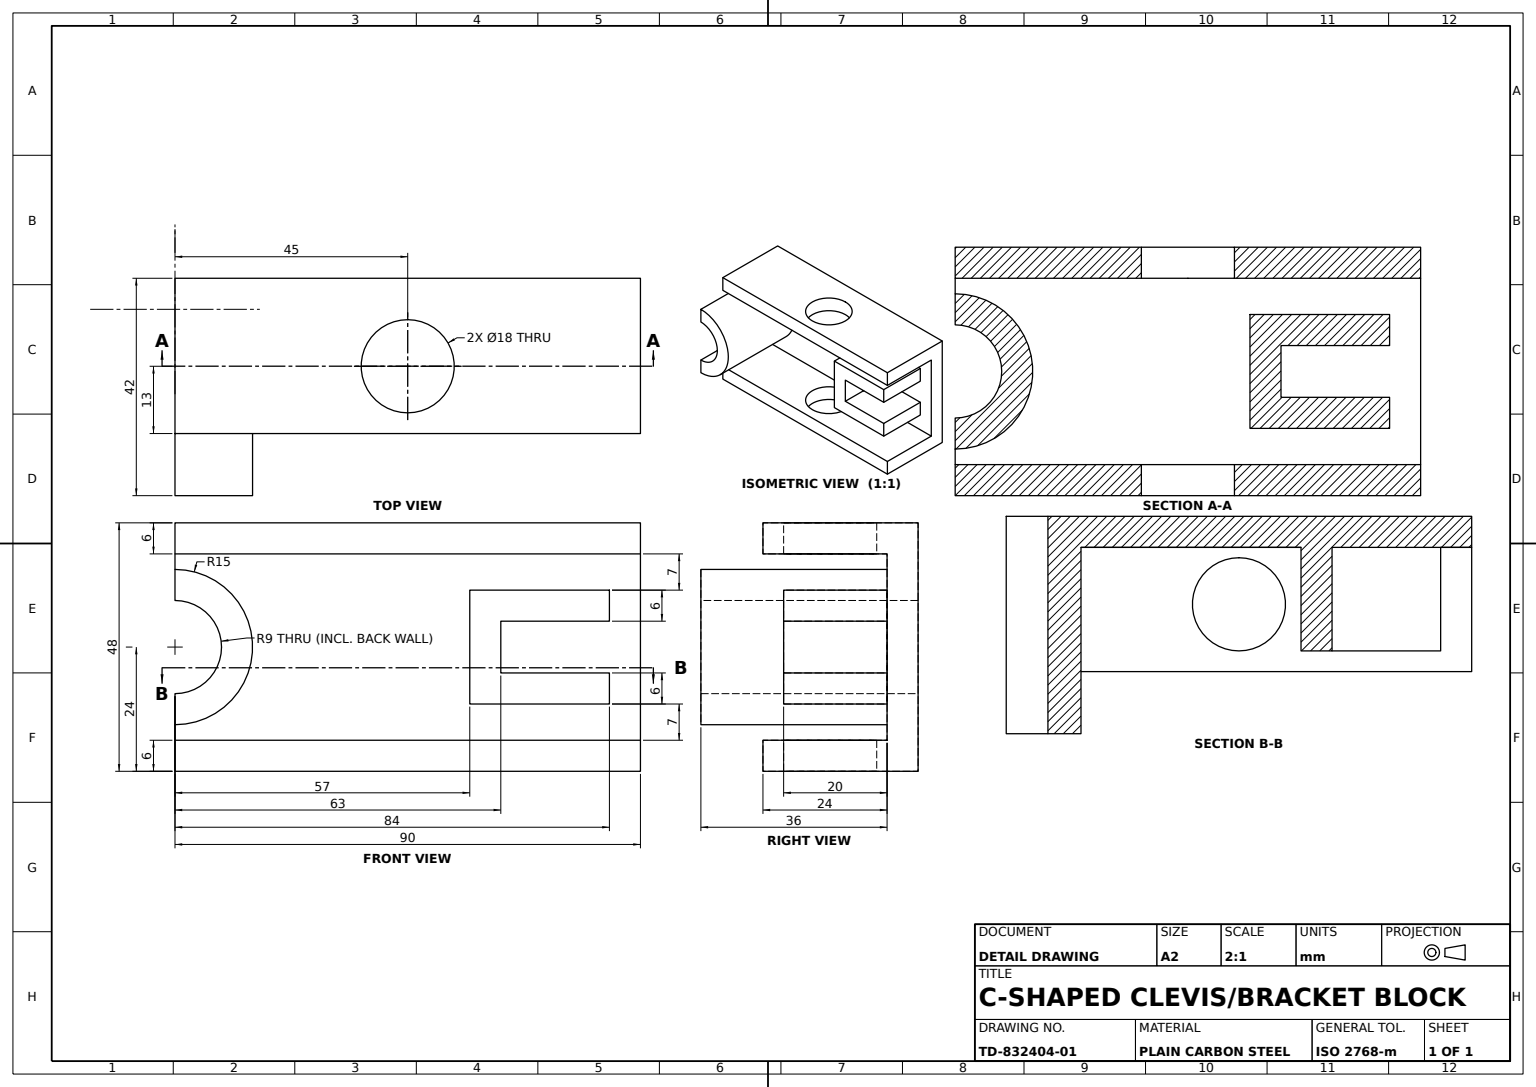
SolidWorks part; units mm, degrees
material "Plain Carbon Steel"
ref_plane "Front Plane" through (0, 0, 0) normal (0, 0, 1) x (1, 0, 0)
ref_plane "Top Plane" through (0, 0, 0) normal (0, 1, 0) x (1, 0, 0)
ref_plane "Right Plane" through (0, 0, 0) normal (1, 0, 0) x (0, 0, -1)
sketch "Base Block Sketch" plane through (0, 0, 0) normal (0, 0, 1) x (1, 0, 0)
  line L0 (0, 0) -> (90, 0)
  line L1 (90, 0) -> (90, 48)
  line L2 (90, 48) -> (0, 48)
  line L3 (0, 48) -> (0, 0)
  dimension "D1" = 90
  dimension "D2" = 48
extrude "Base Block" add sketch "Base Block Sketch" along normal blind 30
sketch "Channel Slot Sketch" plane through (0, 0, 30) normal (0, 0, 1) x (1, 0, 0)
  line L0 (6, 42) -> (6, 6)
  line L1 (0, 48) -> (0, 0) construction
  line L2 (0, 0) -> (90, 0) construction
  line L8 (84, 42) -> (6, 42)
  line L10 (6, 6) -> (84, 6)
  line L11 (84, 6) -> (84, 42)
  dimension "D1" = 6
  dimension "D2" = 84
  dimension "D3" = 6
  dimension "D4" = 42
extrude "Channel Slot" cut sketch "Channel Slot Sketch" against normal blind 24
sketch "Channel Relief Cut 1 Sketch" plane through (0, 0, 30) normal (0, 0, 1) x (1, 0, 0)
  line L0 (6, 42) -> (0, 42)
  line L1 (0, 48) -> (0, 0) construction
  line L2 (0, 42) -> (0, 6)
  line L3 (0, 6) -> (6, 6)
  line L4 (6, 6) -> (6, 42)
extrude "Channel Relief Cut 1" cut sketch "Channel Relief Cut 1 Sketch" against normal blind 24
sketch "Channel Relief Cut 2 Sketch" plane through (0, 0, 30) normal (0, 0, 1) x (1, 0, 0)
  line L0 (84, 42) -> (84, 6)
  line L1 (84, 6) -> (90, 6)
  line L2 (90, 0) -> (90, 48) construction
  line L3 (90, 6) -> (90, 42)
  line L4 (90, 42) -> (84, 42)
extrude "Channel Relief Cut 2" cut sketch "Channel Relief Cut 2 Sketch" against normal blind 24
sketch "Half Cylinder Boss Sketch" plane through (0, 0, 6) normal (0, 0, 1) x (1, 0, 0)
  line L0 (0, 42) -> (0, 6) construction
  line L1 (0, 39) -> (0, 9)
  arc A0 (0, 9) -> (0, 39) centre (0, 24) ccw
  dimension "D1" = 30
  dimension "D2" = 15
extrude "Half Cylinder Boss" add sketch "Half Cylinder Boss Sketch" along normal blind 36
sketch "Boss Bore Sketch" plane through (0, 0, 42) normal (0, 0, 1) x (1, 0, 0)
  line L0 (0, 39) -> (0, 9) construction
  line L1 (0, 33) -> (0, 15)
  arc A0 (0, 15) -> (0, 33) centre (0, 24) ccw
  dimension "D1" = 18
  dimension "D2" = 9
extrude "Boss Bore Ø18" cut sketch "Boss Bore Sketch" against normal blind 42
sketch "Upper Plate Hole Sketch" plane through (0, 0, 0) normal (0, -1, 0) x (1, 0, 0)
  line L0 (0, 30) -> (90, 30) construction
  line L1 (90, 30) -> (90, 0) construction
  circle A0 centre (45, 17) radius 9
  dimension "D1" = 18
  dimension "D4" = 18
  dimension "D2" = 13
  dimension "D3" = 45
extrude "Upper Plate Hole Ø18" cut sketch "Upper Plate Hole Sketch" against normal blind 6
sketch "Lower Plate Hole Sketch" plane through (0, 48, 0) normal (0, 1, 0) x (1, 0, 0)
  line L0 (0, -30) -> (0, 0) construction
  line L1 (90, -30) -> (0, -30) construction
  circle A0 centre (45, -17) radius 9
  dimension "D1" = 18
  dimension "D3" = 18
  dimension "D2" = 13
  dimension "D4" = 45
extrude "Lower Plate Hole Ø18" cut sketch "Lower Plate Hole Sketch" against normal blind 6
sketch "C Clip Boss Sketch" plane through (0, 0, 6) normal (0, 0, 1) x (1, 0, 0)
  line L0 (84, 35) -> (84, 29)
  line L1 (0, 42) -> (0, 39) construction
  line L3 (84, 35) -> (57, 35)
  line L4 (57, 35) -> (57, 13)
  line L5 (57, 13) -> (84, 13)
  line L6 (84, 29) -> (63, 29)
  line L8 (84, 19) -> (63, 19)
  line L9 (63, 19) -> (63, 29)
  line L10 (84, 19) -> (84, 13)
  dimension "D1" = 57
  dimension "D2" = 63
  dimension "D3" = 84
  dimension "D4" = 7
  dimension "D5" = 13
  dimension "D6" = 23
extrude "C Clip Boss" add sketch "C Clip Boss Sketch" along normal blind 20
